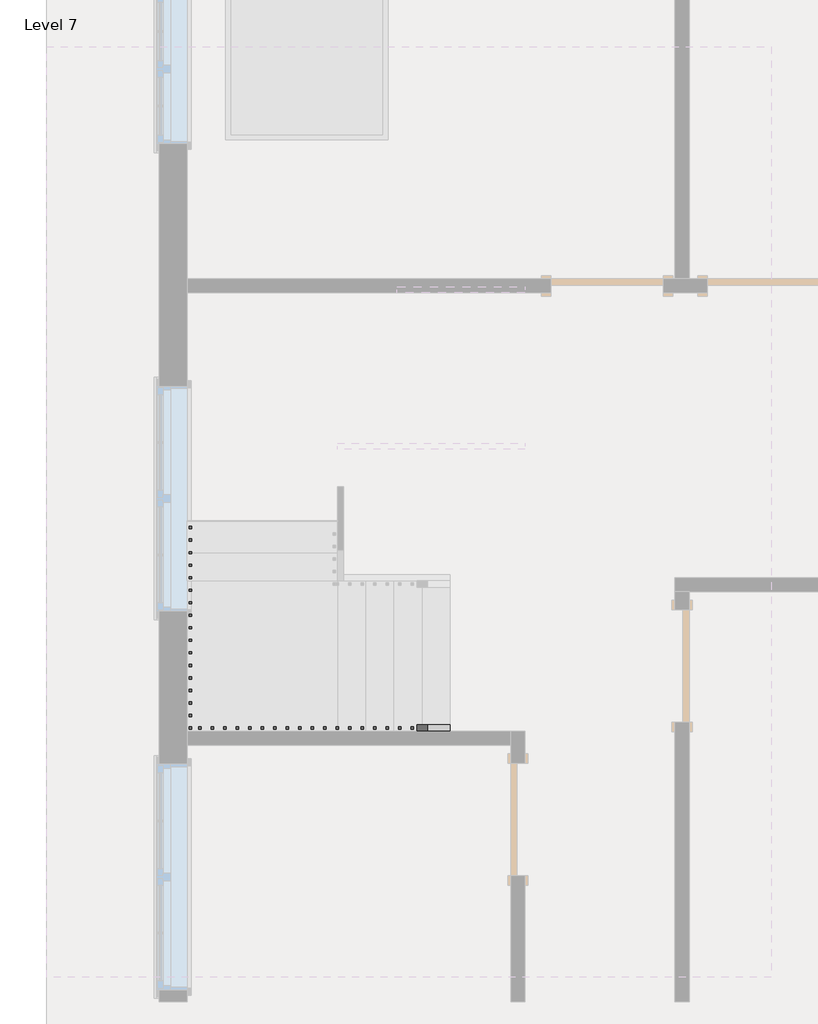
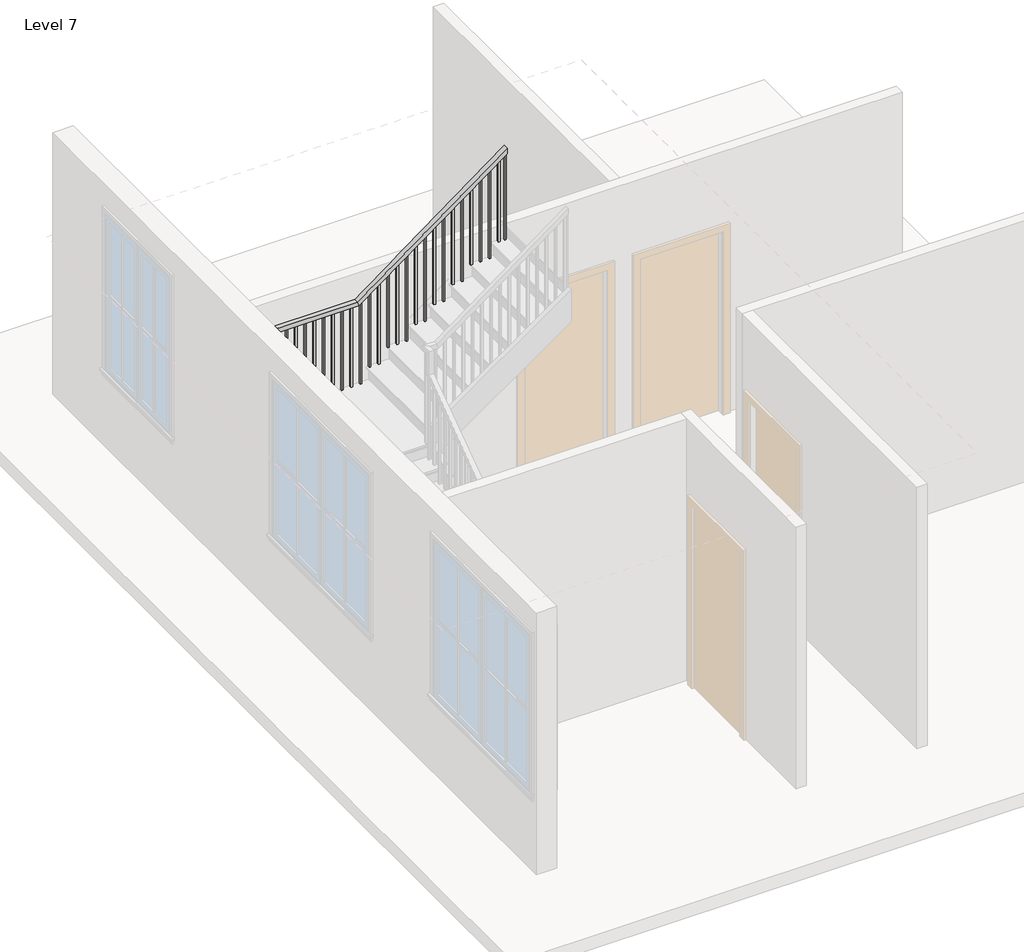
# One storey, part 2 of 3: 1 railing.
"""IFC4 building model written with IfcOpenShell, lengths in millimetres."""

from ifc_helpers import new_model, si_unit, frame, origin, place, context, project, spatial, polyline, outline, extrude, faceted_brep, element, save

model = new_model("IFC4")

# Units and contexts
model_context = context("Model", 3, world=origin())
ifc_project = project(units=[si_unit("LENGTHUNIT", "METRE", prefix="MILLI")], contexts=[model_context])

# Site, building, storey
site = spatial("IfcSite", under=ifc_project)
building = spatial("IfcBuilding", under=site)
storey = spatial("IfcBuildingStorey", under=building, Name="Level 7", Elevation=19050.0)

# Railing
placement = place(None, origin())
element("IfcRailing", 1, ObjectType="Handrail - Rectangular", at=placement, inside=storey, context=model_context, shape_type="SolidModel", body=[
    faceted_brep([(-2683.1105391, -2741.0373761, 20124.8210526), (-2683.1105391, -2741.0373761, 20062.7605986), (-2683.1105391, -2690.2373761, 20062.7605986), (-2683.1105391, -2690.2373761, 20124.8210526), (-3698.24463, -2741.0373761, 20837.1958533), (-3714.290777, -2741.0373761, 20786.3958533), (-3714.290777, -2690.2373761, 20786.3958533), (-3698.24463, -2690.2373761, 20837.1958533), (-4816.7105391, -2741.0373761, 20837.1958533), (-4816.7105391, -2741.0373761, 20786.3958533), (-4765.9105391, -2690.2373761, 20786.3958533), (-4765.9105391, -2690.2373761, 20837.1958533), (-4816.7105391, -1646.8618205, 20837.1958533), (-4816.7105391, -1630.5188912, 20786.3958533), (-4765.9105391, -1630.5188912, 20786.3958533), (-4765.9105391, -1646.8618205, 20837.1958533), (-4816.7105391, -308.3947094, 21797.8181818), (-4816.7105391, -292.0517801, 21747.0181818), (-4765.9105391, -292.0517801, 21747.0181818), (-4765.9105391, -308.3947094, 21797.8181818), (-4816.7105391, 814.9626239, 21797.8181818), (-4816.7105391, 814.9626239, 21747.0181818), (-4765.9105391, 764.1626239, 21747.0181818), (-4765.9105391, 764.1626239, 21797.8181818), (-3721.871578, 814.9626239, 21797.8181818), (-3705.1770744, 814.9626239, 21747.0181818), (-3705.1770744, 764.1626239, 21747.0181818), (-3721.871578, 764.1626239, 21797.8181818), (-2073.5105391, 814.9626239, 23012.4), (-2073.5105391, 764.1626239, 23012.4), (-2073.5105391, 764.1626239, 22949.2987868), (-2073.5105391, 814.9626239, 22949.2987868)], [[[0, 1, 2, 3]], [[1, 0, 4, 5]], [[2, 1, 5, 6]], [[3, 2, 6, 7]], [[0, 3, 7, 4]], [[5, 4, 8, 9]], [[6, 5, 9, 10]], [[7, 6, 10, 11]], [[4, 7, 11, 8]], [[9, 8, 12, 13]], [[10, 9, 13, 14]], [[11, 10, 14, 15]], [[8, 11, 15, 12]], [[13, 12, 16, 17]], [[14, 13, 17, 18]], [[15, 14, 18, 19]], [[12, 15, 19, 16]], [[17, 16, 20, 21]], [[18, 17, 21, 22]], [[19, 18, 22, 23]], [[16, 19, 23, 20]], [[21, 20, 24, 25]], [[22, 21, 25, 26]], [[23, 22, 26, 27]], [[20, 23, 27, 24]], [[28, 29, 30, 31]], [[25, 24, 28, 31]], [[26, 25, 31, 30]], [[27, 26, 30, 29]], [[24, 27, 29, 28]]]),
    extrude(outline(polyline([(22886.1329974, -2159.2355391), (21937.5789474, -2159.2355391), (21937.5789474, -2140.1855391), (22900.1698395, -2140.1855391), (22886.1329974, -2159.2355391)])), frame((0.0, 780.0376239, 0.0), z_axis=(0.0, 1.0, 0.0), x_axis=(0.0, 0.0, 1.0)), (0.0, 0.0, 1.0), 19.05),
    extrude(outline(polyline([(22811.2698395, -2260.8355391), (21777.1578947, -2260.8355391), (21777.1578947, -2241.7855391), (22825.3066816, -2241.7855391), (22811.2698395, -2260.8355391)])), frame((0.0, 780.0376239, 0.0), z_axis=(0.0, 1.0, 0.0), x_axis=(0.0, 0.0, 1.0)), (0.0, 0.0, 1.0), 19.05),
    extrude(outline(polyline([(22736.4066816, -2362.4355391), (21777.1578947, -2362.4355391), (21777.1578947, -2343.3855391), (22750.4435237, -2343.3855391), (22736.4066816, -2362.4355391)])), frame((0.0, 780.0376239, 0.0), z_axis=(0.0, 1.0, 0.0), x_axis=(0.0, 0.0, 1.0)), (0.0, 0.0, 1.0), 19.05),
    extrude(outline(polyline([(22661.5435237, -2464.0355391), (21777.1578947, -2464.0355391), (21777.1578947, -2444.9855391), (22675.5803658, -2444.9855391), (22661.5435237, -2464.0355391)])), frame((0.0, 780.0376239, 0.0), z_axis=(0.0, 1.0, 0.0), x_axis=(0.0, 0.0, 1.0)), (0.0, 0.0, 1.0), 19.05),
    extrude(outline(polyline([(22586.6803658, -2565.6355391), (21616.7368421, -2565.6355391), (21616.7368421, -2546.5855391), (22600.7172079, -2546.5855391), (22586.6803658, -2565.6355391)])), frame((0.0, 780.0376239, 0.0), z_axis=(0.0, 1.0, 0.0), x_axis=(0.0, 0.0, 1.0)), (0.0, 0.0, 1.0), 19.05),
    extrude(outline(polyline([(22511.8172079, -2667.2355391), (21616.7368421, -2667.2355391), (21616.7368421, -2648.1855391), (22525.85405, -2648.1855391), (22511.8172079, -2667.2355391)])), frame((0.0, 780.0376239, 0.0), z_axis=(0.0, 1.0, 0.0), x_axis=(0.0, 0.0, 1.0)), (0.0, 0.0, 1.0), 19.05),
    extrude(outline(polyline([(22436.95405, -2768.8355391), (21456.3157895, -2768.8355391), (21456.3157895, -2749.7855391), (22450.9908921, -2749.7855391), (22436.95405, -2768.8355391)])), frame((0.0, 780.0376239, 0.0), z_axis=(0.0, 1.0, 0.0), x_axis=(0.0, 0.0, 1.0)), (0.0, 0.0, 1.0), 19.05),
    extrude(outline(polyline([(22362.0908921, -2870.4355391), (21456.3157895, -2870.4355391), (21456.3157895, -2851.3855391), (22376.1277342, -2851.3855391), (22362.0908921, -2870.4355391)])), frame((0.0, 780.0376239, 0.0), z_axis=(0.0, 1.0, 0.0), x_axis=(0.0, 0.0, 1.0)), (0.0, 0.0, 1.0), 19.05),
    extrude(outline(polyline([(22287.2277342, -2972.0355391), (21295.8947368, -2972.0355391), (21295.8947368, -2952.9855391), (22301.2645763, -2952.9855391), (22287.2277342, -2972.0355391)])), frame((0.0, 780.0376239, 0.0), z_axis=(0.0, 1.0, 0.0), x_axis=(0.0, 0.0, 1.0)), (0.0, 0.0, 1.0), 19.05),
    extrude(outline(polyline([(22212.3645763, -3073.6355391), (21295.8947368, -3073.6355391), (21295.8947368, -3054.5855391), (22226.4014184, -3054.5855391), (22212.3645763, -3073.6355391)])), frame((0.0, 780.0376239, 0.0), z_axis=(0.0, 1.0, 0.0), x_axis=(0.0, 0.0, 1.0)), (0.0, 0.0, 1.0), 19.05),
    extrude(outline(polyline([(22137.5014184, -3175.2355391), (21135.4736842, -3175.2355391), (21135.4736842, -3156.1855391), (22151.5382605, -3156.1855391), (22137.5014184, -3175.2355391)])), frame((0.0, 780.0376239, 0.0), z_axis=(0.0, 1.0, 0.0), x_axis=(0.0, 0.0, 1.0)), (0.0, 0.0, 1.0), 19.05),
    extrude(outline(polyline([(22062.6382605, -3276.8355391), (21135.4736842, -3276.8355391), (21135.4736842, -3257.7855391), (22076.6751026, -3257.7855391), (22062.6382605, -3276.8355391)])), frame((0.0, 780.0376239, 0.0), z_axis=(0.0, 1.0, 0.0), x_axis=(0.0, 0.0, 1.0)), (0.0, 0.0, 1.0), 19.05),
    extrude(outline(polyline([(21987.7751026, -3378.4355391), (21135.4736842, -3378.4355391), (21135.4736842, -3359.3855391), (22001.8119447, -3359.3855391), (21987.7751026, -3378.4355391)])), frame((0.0, 780.0376239, 0.0), z_axis=(0.0, 1.0, 0.0), x_axis=(0.0, 0.0, 1.0)), (0.0, 0.0, 1.0), 19.05),
    extrude(outline(polyline([(21912.9119447, -3480.0355391), (20975.0526316, -3480.0355391), (20975.0526316, -3460.9855391), (21926.9487868, -3460.9855391), (21912.9119447, -3480.0355391)])), frame((0.0, 780.0376239, 0.0), z_axis=(0.0, 1.0, 0.0), x_axis=(0.0, 0.0, 1.0)), (0.0, 0.0, 1.0), 19.05),
    extrude(outline(polyline([(21838.0487868, -3581.6355391), (20975.0526316, -3581.6355391), (20975.0526316, -3562.5855391), (21852.0856289, -3562.5855391), (21838.0487868, -3581.6355391)])), frame((0.0, 780.0376239, 0.0), z_axis=(0.0, 1.0, 0.0), x_axis=(0.0, 0.0, 1.0)), (0.0, 0.0, 1.0), 19.05),
    extrude(outline(polyline([(21763.1856289, -3683.2355391), (20814.6315789, -3683.2355391), (20814.6315789, -3664.1855391), (21777.222471, -3664.1855391), (21763.1856289, -3683.2355391)])), frame((0.0, 780.0376239, 0.0), z_axis=(0.0, 1.0, 0.0), x_axis=(0.0, 0.0, 1.0)), (0.0, 0.0, 1.0), 19.05),
    extrude(outline(polyline([(-3784.8355391, 799.0876239), (-3765.7855391, 799.0876239), (-3765.7855391, 780.0376239), (-3784.8355391, 780.0376239), (-3784.8355391, 799.0876239)])), frame((0.0, 0.0, 20814.6315789), z_axis=(0.0, 0.0, 1.0), x_axis=(1.0, 0.0, 0.0)), (0.0, 0.0, 1.0), 932.3866029),
    extrude(outline(polyline([(-3886.4355391, 799.0876239), (-3867.3855391, 799.0876239), (-3867.3855391, 780.0376239), (-3886.4355391, 780.0376239), (-3886.4355391, 799.0876239)])), frame((0.0, 0.0, 20814.6315789), z_axis=(0.0, 0.0, 1.0), x_axis=(1.0, 0.0, 0.0)), (0.0, 0.0, 1.0), 932.3866029),
    extrude(outline(polyline([(-3988.0355391, 799.0876239), (-3968.9855391, 799.0876239), (-3968.9855391, 780.0376239), (-3988.0355391, 780.0376239), (-3988.0355391, 799.0876239)])), frame((0.0, 0.0, 20814.6315789), z_axis=(0.0, 0.0, 1.0), x_axis=(1.0, 0.0, 0.0)), (0.0, 0.0, 1.0), 932.3866029),
    extrude(outline(polyline([(-4089.6355391, 799.0876239), (-4070.5855391, 799.0876239), (-4070.5855391, 780.0376239), (-4089.6355391, 780.0376239), (-4089.6355391, 799.0876239)])), frame((0.0, 0.0, 20814.6315789), z_axis=(0.0, 0.0, 1.0), x_axis=(1.0, 0.0, 0.0)), (0.0, 0.0, 1.0), 932.3866029),
    extrude(outline(polyline([(-4191.2355391, 799.0876239), (-4172.1855391, 799.0876239), (-4172.1855391, 780.0376239), (-4191.2355391, 780.0376239), (-4191.2355391, 799.0876239)])), frame((0.0, 0.0, 20814.6315789), z_axis=(0.0, 0.0, 1.0), x_axis=(1.0, 0.0, 0.0)), (0.0, 0.0, 1.0), 932.3866029),
    extrude(outline(polyline([(-4292.8355391, 799.0876239), (-4273.7855391, 799.0876239), (-4273.7855391, 780.0376239), (-4292.8355391, 780.0376239), (-4292.8355391, 799.0876239)])), frame((0.0, 0.0, 20814.6315789), z_axis=(0.0, 0.0, 1.0), x_axis=(1.0, 0.0, 0.0)), (0.0, 0.0, 1.0), 932.3866029),
    extrude(outline(polyline([(-4394.4355391, 799.0876239), (-4375.3855391, 799.0876239), (-4375.3855391, 780.0376239), (-4394.4355391, 780.0376239), (-4394.4355391, 799.0876239)])), frame((0.0, 0.0, 20814.6315789), z_axis=(0.0, 0.0, 1.0), x_axis=(1.0, 0.0, 0.0)), (0.0, 0.0, 1.0), 932.3866029),
    extrude(outline(polyline([(-4496.0355391, 799.0876239), (-4476.9855391, 799.0876239), (-4476.9855391, 780.0376239), (-4496.0355391, 780.0376239), (-4496.0355391, 799.0876239)])), frame((0.0, 0.0, 20814.6315789), z_axis=(0.0, 0.0, 1.0), x_axis=(1.0, 0.0, 0.0)), (0.0, 0.0, 1.0), 932.3866029),
    extrude(outline(polyline([(-4597.6355391, 799.0876239), (-4578.5855391, 799.0876239), (-4578.5855391, 780.0376239), (-4597.6355391, 780.0376239), (-4597.6355391, 799.0876239)])), frame((0.0, 0.0, 20814.6315789), z_axis=(0.0, 0.0, 1.0), x_axis=(1.0, 0.0, 0.0)), (0.0, 0.0, 1.0), 932.3866029),
    extrude(outline(polyline([(-4699.2355391, 799.0876239), (-4680.1855391, 799.0876239), (-4680.1855391, 780.0376239), (-4699.2355391, 780.0376239), (-4699.2355391, 799.0876239)])), frame((0.0, 0.0, 20814.6315789), z_axis=(0.0, 0.0, 1.0), x_axis=(1.0, 0.0, 0.0)), (0.0, 0.0, 1.0), 932.3866029),
    extrude(outline(polyline([(-4800.8355391, 729.2376239), (-4800.8355391, 748.2876239), (-4781.7855391, 748.2876239), (-4781.7855391, 729.2376239), (-4800.8355391, 729.2376239)])), frame((0.0, 0.0, 20814.6315789), z_axis=(0.0, 0.0, 1.0), x_axis=(1.0, 0.0, 0.0)), (0.0, 0.0, 1.0), 932.3866029),
    extrude(outline(polyline([(-4800.8355391, 627.6376239), (-4800.8355391, 646.6876239), (-4781.7855391, 646.6876239), (-4781.7855391, 627.6376239), (-4800.8355391, 627.6376239)])), frame((0.0, 0.0, 20814.6315789), z_axis=(0.0, 0.0, 1.0), x_axis=(1.0, 0.0, 0.0)), (0.0, 0.0, 1.0), 932.3866029),
    extrude(outline(polyline([(-4800.8355391, 526.0376239), (-4800.8355391, 545.0876239), (-4781.7855391, 545.0876239), (-4781.7855391, 526.0376239), (-4800.8355391, 526.0376239)])), frame((0.0, 0.0, 20814.6315789), z_axis=(0.0, 0.0, 1.0), x_axis=(1.0, 0.0, 0.0)), (0.0, 0.0, 1.0), 932.3866029),
    extrude(outline(polyline([(-4800.8355391, 424.4376239), (-4800.8355391, 443.4876239), (-4781.7855391, 443.4876239), (-4781.7855391, 424.4376239), (-4800.8355391, 424.4376239)])), frame((0.0, 0.0, 20814.6315789), z_axis=(0.0, 0.0, 1.0), x_axis=(1.0, 0.0, 0.0)), (0.0, 0.0, 1.0), 932.3866029),
    extrude(outline(polyline([(-4800.8355391, 322.8376239), (-4800.8355391, 341.8876239), (-4781.7855391, 341.8876239), (-4781.7855391, 322.8376239), (-4800.8355391, 322.8376239)])), frame((0.0, 0.0, 20814.6315789), z_axis=(0.0, 0.0, 1.0), x_axis=(1.0, 0.0, 0.0)), (0.0, 0.0, 1.0), 932.3866029),
    extrude(outline(polyline([(-4800.8355391, 221.2376239), (-4800.8355391, 240.2876239), (-4781.7855391, 240.2876239), (-4781.7855391, 221.2376239), (-4800.8355391, 221.2376239)])), frame((0.0, 0.0, 20814.6315789), z_axis=(0.0, 0.0, 1.0), x_axis=(1.0, 0.0, 0.0)), (0.0, 0.0, 1.0), 932.3866029),
    extrude(outline(polyline([(-4800.8355391, 119.6376239), (-4800.8355391, 138.6876239), (-4781.7855391, 138.6876239), (-4781.7855391, 119.6376239), (-4800.8355391, 119.6376239)])), frame((0.0, 0.0, 20814.6315789), z_axis=(0.0, 0.0, 1.0), x_axis=(1.0, 0.0, 0.0)), (0.0, 0.0, 1.0), 932.3866029),
    extrude(outline(polyline([(-4800.8355391, 18.0376239), (-4800.8355391, 37.0876239), (-4781.7855391, 37.0876239), (-4781.7855391, 18.0376239), (-4800.8355391, 18.0376239)])), frame((0.0, 0.0, 20814.6315789), z_axis=(0.0, 0.0, 1.0), x_axis=(1.0, 0.0, 0.0)), (0.0, 0.0, 1.0), 932.3866029),
    extrude(outline(polyline([(-4800.8355391, -83.5623761), (-4800.8355391, -64.5123761), (-4781.7855391, -64.5123761), (-4781.7855391, -83.5623761), (-4800.8355391, -83.5623761)])), frame((0.0, 0.0, 20814.6315789), z_axis=(0.0, 0.0, 1.0), x_axis=(1.0, 0.0, 0.0)), (0.0, 0.0, 1.0), 932.3866029),
    extrude(outline(polyline([(-4800.8355391, -185.1623761), (-4800.8355391, -166.1123761), (-4781.7855391, -166.1123761), (-4781.7855391, -185.1623761), (-4800.8355391, -185.1623761)])), frame((0.0, 0.0, 20814.6315789), z_axis=(0.0, 0.0, 1.0), x_axis=(1.0, 0.0, 0.0)), (0.0, 0.0, 1.0), 932.3866029),
    extrude(outline(polyline([(-4800.8355391, -286.7623761), (-4800.8355391, -267.7123761), (-4781.7855391, -267.7123761), (-4781.7855391, -286.7623761), (-4800.8355391, -286.7623761)])), frame((0.0, 0.0, 20814.6315789), z_axis=(0.0, 0.0, 1.0), x_axis=(1.0, 0.0, 0.0)), (0.0, 0.0, 1.0), 932.3866029),
    extrude(outline(polyline([(-369.3123761, 21691.5679933), (-369.3123761, 20814.6315789), (-388.3623761, 20814.6315789), (-388.3623761, 21677.8957445), (-369.3123761, 21691.5679933)])), frame((-4800.8355391, 0.0, 0.0), z_axis=(1.0, 0.0, 0.0), x_axis=(0.0, 1.0, 0.0)), (0.0, 0.0, 1.0), 19.05),
    extrude(outline(polyline([(-470.9123761, 21618.649333), (-470.9123761, 20654.2105263), (-489.9623761, 20654.2105263), (-489.9623761, 21604.9770842), (-470.9123761, 21618.649333)])), frame((-4800.8355391, 0.0, 0.0), z_axis=(1.0, 0.0, 0.0), x_axis=(0.0, 1.0, 0.0)), (0.0, 0.0, 1.0), 19.05),
    extrude(outline(polyline([(-572.5123761, 21545.7306727), (-572.5123761, 20654.2105263), (-591.5623761, 20654.2105263), (-591.5623761, 21532.0584239), (-572.5123761, 21545.7306727)])), frame((-4800.8355391, 0.0, 0.0), z_axis=(1.0, 0.0, 0.0), x_axis=(0.0, 1.0, 0.0)), (0.0, 0.0, 1.0), 19.05),
    extrude(outline(polyline([(-674.1123761, 21472.8120124), (-674.1123761, 20493.7894737), (-693.1623761, 20493.7894737), (-693.1623761, 21459.1397636), (-674.1123761, 21472.8120124)])), frame((-4800.8355391, 0.0, 0.0), z_axis=(1.0, 0.0, 0.0), x_axis=(0.0, 1.0, 0.0)), (0.0, 0.0, 1.0), 19.05),
    extrude(outline(polyline([(-775.7123761, 21399.8933521), (-775.7123761, 20493.7894737), (-794.7623761, 20493.7894737), (-794.7623761, 21386.2211033), (-775.7123761, 21399.8933521)])), frame((-4800.8355391, 0.0, 0.0), z_axis=(1.0, 0.0, 0.0), x_axis=(0.0, 1.0, 0.0)), (0.0, 0.0, 1.0), 19.05),
    extrude(outline(polyline([(-877.3123761, 21326.9746919), (-877.3123761, 20333.3684211), (-896.3623761, 20333.3684211), (-896.3623761, 21313.302443), (-877.3123761, 21326.9746919)])), frame((-4800.8355391, 0.0, 0.0), z_axis=(1.0, 0.0, 0.0), x_axis=(0.0, 1.0, 0.0)), (0.0, 0.0, 1.0), 19.05),
    extrude(outline(polyline([(-978.9123761, 21254.0560316), (-978.9123761, 20333.3684211), (-997.9623761, 20333.3684211), (-997.9623761, 21240.3837828), (-978.9123761, 21254.0560316)])), frame((-4800.8355391, 0.0, 0.0), z_axis=(1.0, 0.0, 0.0), x_axis=(0.0, 1.0, 0.0)), (0.0, 0.0, 1.0), 19.05),
    extrude(outline(polyline([(-1080.5123761, 21181.1373713), (-1080.5123761, 20172.9473684), (-1099.5623761, 20172.9473684), (-1099.5623761, 21167.4651225), (-1080.5123761, 21181.1373713)])), frame((-4800.8355391, 0.0, 0.0), z_axis=(1.0, 0.0, 0.0), x_axis=(0.0, 1.0, 0.0)), (0.0, 0.0, 1.0), 19.05),
    extrude(outline(polyline([(-1182.1123761, 21108.218711), (-1182.1123761, 20172.9473684), (-1201.1623761, 20172.9473684), (-1201.1623761, 21094.5464622), (-1182.1123761, 21108.218711)])), frame((-4800.8355391, 0.0, 0.0), z_axis=(1.0, 0.0, 0.0), x_axis=(0.0, 1.0, 0.0)), (0.0, 0.0, 1.0), 19.05),
    extrude(outline(polyline([(-1283.7123761, 21035.3000507), (-1283.7123761, 20172.9473684), (-1302.7623761, 20172.9473684), (-1302.7623761, 21021.6278019), (-1283.7123761, 21035.3000507)])), frame((-4800.8355391, 0.0, 0.0), z_axis=(1.0, 0.0, 0.0), x_axis=(0.0, 1.0, 0.0)), (0.0, 0.0, 1.0), 19.05),
    extrude(outline(polyline([(-1385.3123761, 20962.3813904), (-1385.3123761, 20012.5263158), (-1404.3623761, 20012.5263158), (-1404.3623761, 20948.7091416), (-1385.3123761, 20962.3813904)])), frame((-4800.8355391, 0.0, 0.0), z_axis=(1.0, 0.0, 0.0), x_axis=(0.0, 1.0, 0.0)), (0.0, 0.0, 1.0), 19.05),
    extrude(outline(polyline([(-1486.9123761, 20889.4627301), (-1486.9123761, 20012.5263158), (-1505.9623761, 20012.5263158), (-1505.9623761, 20875.7904813), (-1486.9123761, 20889.4627301)])), frame((-4800.8355391, 0.0, 0.0), z_axis=(1.0, 0.0, 0.0), x_axis=(0.0, 1.0, 0.0)), (0.0, 0.0, 1.0), 19.05),
    extrude(outline(polyline([(-1588.5123761, 20816.5440698), (-1588.5123761, 19852.1052632), (-1607.5623761, 19852.1052632), (-1607.5623761, 20802.871821), (-1588.5123761, 20816.5440698)])), frame((-4800.8355391, 0.0, 0.0), z_axis=(1.0, 0.0, 0.0), x_axis=(0.0, 1.0, 0.0)), (0.0, 0.0, 1.0), 19.05),
    extrude(outline(polyline([(-4800.8355391, -1709.1623761), (-4800.8355391, -1690.1123761), (-4781.7855391, -1690.1123761), (-4781.7855391, -1709.1623761), (-4800.8355391, -1709.1623761)])), frame((0.0, 0.0, 19852.1052632), z_axis=(0.0, 0.0, 1.0), x_axis=(1.0, 0.0, 0.0)), (0.0, 0.0, 1.0), 934.2905901),
    extrude(outline(polyline([(-4800.8355391, -1810.7623761), (-4800.8355391, -1791.7123761), (-4781.7855391, -1791.7123761), (-4781.7855391, -1810.7623761), (-4800.8355391, -1810.7623761)])), frame((0.0, 0.0, 19852.1052632), z_axis=(0.0, 0.0, 1.0), x_axis=(1.0, 0.0, 0.0)), (0.0, 0.0, 1.0), 934.2905901),
    extrude(outline(polyline([(-4800.8355391, -1912.3623761), (-4800.8355391, -1893.3123761), (-4781.7855391, -1893.3123761), (-4781.7855391, -1912.3623761), (-4800.8355391, -1912.3623761)])), frame((0.0, 0.0, 19852.1052632), z_axis=(0.0, 0.0, 1.0), x_axis=(1.0, 0.0, 0.0)), (0.0, 0.0, 1.0), 934.2905901),
    extrude(outline(polyline([(-4800.8355391, -2013.9623761), (-4800.8355391, -1994.9123761), (-4781.7855391, -1994.9123761), (-4781.7855391, -2013.9623761), (-4800.8355391, -2013.9623761)])), frame((0.0, 0.0, 19852.1052632), z_axis=(0.0, 0.0, 1.0), x_axis=(1.0, 0.0, 0.0)), (0.0, 0.0, 1.0), 934.2905901),
    extrude(outline(polyline([(-4800.8355391, -2115.5623761), (-4800.8355391, -2096.5123761), (-4781.7855391, -2096.5123761), (-4781.7855391, -2115.5623761), (-4800.8355391, -2115.5623761)])), frame((0.0, 0.0, 19852.1052632), z_axis=(0.0, 0.0, 1.0), x_axis=(1.0, 0.0, 0.0)), (0.0, 0.0, 1.0), 934.2905901),
    extrude(outline(polyline([(-4800.8355391, -2217.1623761), (-4800.8355391, -2198.1123761), (-4781.7855391, -2198.1123761), (-4781.7855391, -2217.1623761), (-4800.8355391, -2217.1623761)])), frame((0.0, 0.0, 19852.1052632), z_axis=(0.0, 0.0, 1.0), x_axis=(1.0, 0.0, 0.0)), (0.0, 0.0, 1.0), 934.2905901),
    extrude(outline(polyline([(-4800.8355391, -2318.7623761), (-4800.8355391, -2299.7123761), (-4781.7855391, -2299.7123761), (-4781.7855391, -2318.7623761), (-4800.8355391, -2318.7623761)])), frame((0.0, 0.0, 19852.1052632), z_axis=(0.0, 0.0, 1.0), x_axis=(1.0, 0.0, 0.0)), (0.0, 0.0, 1.0), 934.2905901),
    extrude(outline(polyline([(-4800.8355391, -2420.3623761), (-4800.8355391, -2401.3123761), (-4781.7855391, -2401.3123761), (-4781.7855391, -2420.3623761), (-4800.8355391, -2420.3623761)])), frame((0.0, 0.0, 19852.1052632), z_axis=(0.0, 0.0, 1.0), x_axis=(1.0, 0.0, 0.0)), (0.0, 0.0, 1.0), 934.2905901),
    extrude(outline(polyline([(-4800.8355391, -2521.9623761), (-4800.8355391, -2502.9123761), (-4781.7855391, -2502.9123761), (-4781.7855391, -2521.9623761), (-4800.8355391, -2521.9623761)])), frame((0.0, 0.0, 19852.1052632), z_axis=(0.0, 0.0, 1.0), x_axis=(1.0, 0.0, 0.0)), (0.0, 0.0, 1.0), 934.2905901),
    extrude(outline(polyline([(-4800.8355391, -2623.5623761), (-4800.8355391, -2604.5123761), (-4781.7855391, -2604.5123761), (-4781.7855391, -2623.5623761), (-4800.8355391, -2623.5623761)])), frame((0.0, 0.0, 19852.1052632), z_axis=(0.0, 0.0, 1.0), x_axis=(1.0, 0.0, 0.0)), (0.0, 0.0, 1.0), 934.2905901),
    extrude(outline(polyline([(-4705.5855391, -2725.1623761), (-4724.6355391, -2725.1623761), (-4724.6355391, -2706.1123761), (-4705.5855391, -2706.1123761), (-4705.5855391, -2725.1623761)])), frame((0.0, 0.0, 19852.1052632), z_axis=(0.0, 0.0, 1.0), x_axis=(1.0, 0.0, 0.0)), (0.0, 0.0, 1.0), 934.2905901),
    extrude(outline(polyline([(-4603.9855391, -2725.1623761), (-4623.0355391, -2725.1623761), (-4623.0355391, -2706.1123761), (-4603.9855391, -2706.1123761), (-4603.9855391, -2725.1623761)])), frame((0.0, 0.0, 19852.1052632), z_axis=(0.0, 0.0, 1.0), x_axis=(1.0, 0.0, 0.0)), (0.0, 0.0, 1.0), 934.2905901),
    extrude(outline(polyline([(-4502.3855391, -2725.1623761), (-4521.4355391, -2725.1623761), (-4521.4355391, -2706.1123761), (-4502.3855391, -2706.1123761), (-4502.3855391, -2725.1623761)])), frame((0.0, 0.0, 19852.1052632), z_axis=(0.0, 0.0, 1.0), x_axis=(1.0, 0.0, 0.0)), (0.0, 0.0, 1.0), 934.2905901),
    extrude(outline(polyline([(-4400.7855391, -2725.1623761), (-4419.8355391, -2725.1623761), (-4419.8355391, -2706.1123761), (-4400.7855391, -2706.1123761), (-4400.7855391, -2725.1623761)])), frame((0.0, 0.0, 19852.1052632), z_axis=(0.0, 0.0, 1.0), x_axis=(1.0, 0.0, 0.0)), (0.0, 0.0, 1.0), 934.2905901),
    extrude(outline(polyline([(-4299.1855391, -2725.1623761), (-4318.2355391, -2725.1623761), (-4318.2355391, -2706.1123761), (-4299.1855391, -2706.1123761), (-4299.1855391, -2725.1623761)])), frame((0.0, 0.0, 19852.1052632), z_axis=(0.0, 0.0, 1.0), x_axis=(1.0, 0.0, 0.0)), (0.0, 0.0, 1.0), 934.2905901),
    extrude(outline(polyline([(-4197.5855391, -2725.1623761), (-4216.6355391, -2725.1623761), (-4216.6355391, -2706.1123761), (-4197.5855391, -2706.1123761), (-4197.5855391, -2725.1623761)])), frame((0.0, 0.0, 19852.1052632), z_axis=(0.0, 0.0, 1.0), x_axis=(1.0, 0.0, 0.0)), (0.0, 0.0, 1.0), 934.2905901),
    extrude(outline(polyline([(-4095.9855391, -2725.1623761), (-4115.0355391, -2725.1623761), (-4115.0355391, -2706.1123761), (-4095.9855391, -2706.1123761), (-4095.9855391, -2725.1623761)])), frame((0.0, 0.0, 19852.1052632), z_axis=(0.0, 0.0, 1.0), x_axis=(1.0, 0.0, 0.0)), (0.0, 0.0, 1.0), 934.2905901),
    extrude(outline(polyline([(-3994.3855391, -2725.1623761), (-4013.4355391, -2725.1623761), (-4013.4355391, -2706.1123761), (-3994.3855391, -2706.1123761), (-3994.3855391, -2725.1623761)])), frame((0.0, 0.0, 19852.1052632), z_axis=(0.0, 0.0, 1.0), x_axis=(1.0, 0.0, 0.0)), (0.0, 0.0, 1.0), 934.2905901),
    extrude(outline(polyline([(-3892.7855391, -2725.1623761), (-3911.8355391, -2725.1623761), (-3911.8355391, -2706.1123761), (-3892.7855391, -2706.1123761), (-3892.7855391, -2725.1623761)])), frame((0.0, 0.0, 19852.1052632), z_axis=(0.0, 0.0, 1.0), x_axis=(1.0, 0.0, 0.0)), (0.0, 0.0, 1.0), 934.2905901),
    extrude(outline(polyline([(-3791.1855391, -2725.1623761), (-3810.2355391, -2725.1623761), (-3810.2355391, -2706.1123761), (-3791.1855391, -2706.1123761), (-3791.1855391, -2725.1623761)])), frame((0.0, 0.0, 19852.1052632), z_axis=(0.0, 0.0, 1.0), x_axis=(1.0, 0.0, 0.0)), (0.0, 0.0, 1.0), 934.2905901),
    extrude(outline(polyline([(-3689.5855391, -2725.1623761), (-3708.6355391, -2725.1623761), (-3708.6355391, -2706.1123761), (-3689.5855391, -2706.1123761), (-3689.5855391, -2725.1623761)])), frame((0.0, 0.0, 19852.1052632), z_axis=(0.0, 0.0, 1.0), x_axis=(1.0, 0.0, 0.0)), (0.0, 0.0, 1.0), 934.2905901),
    extrude(outline(polyline([(20711.1290196, -3607.0355391), (19852.1052632, -3607.0355391), (19852.1052632, -3587.9855391), (20697.7605986, -3587.9855391), (20711.1290196, -3607.0355391)])), frame((0.0, -2725.1623761, 0.0), z_axis=(0.0, 1.0, 0.0), x_axis=(0.0, 0.0, 1.0)), (0.0, 0.0, 1.0), 19.05),
    extrude(outline(polyline([(20639.830774, -3505.4355391), (19691.6842105, -3505.4355391), (19691.6842105, -3486.3855391), (20626.462353, -3486.3855391), (20639.830774, -3505.4355391)])), frame((0.0, -2725.1623761, 0.0), z_axis=(0.0, 1.0, 0.0), x_axis=(0.0, 0.0, 1.0)), (0.0, 0.0, 1.0), 19.05),
    extrude(outline(polyline([(20568.5325284, -3403.8355391), (19691.6842105, -3403.8355391), (19691.6842105, -3384.7855391), (20555.1641074, -3384.7855391), (20568.5325284, -3403.8355391)])), frame((0.0, -2725.1623761, 0.0), z_axis=(0.0, 1.0, 0.0), x_axis=(0.0, 0.0, 1.0)), (0.0, 0.0, 1.0), 19.05),
    extrude(outline(polyline([(20497.2342828, -3302.2355391), (19531.2631579, -3302.2355391), (19531.2631579, -3283.1855391), (20483.8658617, -3283.1855391), (20497.2342828, -3302.2355391)])), frame((0.0, -2725.1623761, 0.0), z_axis=(0.0, 1.0, 0.0), x_axis=(0.0, 0.0, 1.0)), (0.0, 0.0, 1.0), 19.05),
    extrude(outline(polyline([(20425.9360372, -3200.6355391), (19531.2631579, -3200.6355391), (19531.2631579, -3181.5855391), (20412.5676161, -3181.5855391), (20425.9360372, -3200.6355391)])), frame((0.0, -2725.1623761, 0.0), z_axis=(0.0, 1.0, 0.0), x_axis=(0.0, 0.0, 1.0)), (0.0, 0.0, 1.0), 19.05),
    extrude(outline(polyline([(20354.6377916, -3099.0355391), (19370.8421053, -3099.0355391), (19370.8421053, -3079.9855391), (20341.2693705, -3079.9855391), (20354.6377916, -3099.0355391)])), frame((0.0, -2725.1623761, 0.0), z_axis=(0.0, 1.0, 0.0), x_axis=(0.0, 0.0, 1.0)), (0.0, 0.0, 1.0), 19.05),
    extrude(outline(polyline([(20283.3395459, -2997.4355391), (19370.8421053, -2997.4355391), (19370.8421053, -2978.3855391), (20269.9711249, -2978.3855391), (20283.3395459, -2997.4355391)])), frame((0.0, -2725.1623761, 0.0), z_axis=(0.0, 1.0, 0.0), x_axis=(0.0, 0.0, 1.0)), (0.0, 0.0, 1.0), 19.05),
    extrude(outline(polyline([(20212.0413003, -2895.8355391), (19210.4210526, -2895.8355391), (19210.4210526, -2876.7855391), (20198.6728793, -2876.7855391), (20212.0413003, -2895.8355391)])), frame((0.0, -2725.1623761, 0.0), z_axis=(0.0, 1.0, 0.0), x_axis=(0.0, 0.0, 1.0)), (0.0, 0.0, 1.0), 19.05),
    extrude(outline(polyline([(20140.7430547, -2794.2355391), (19210.4210526, -2794.2355391), (19210.4210526, -2775.1855391), (20127.3746337, -2775.1855391), (20140.7430547, -2794.2355391)])), frame((0.0, -2725.1623761, 0.0), z_axis=(0.0, 1.0, 0.0), x_axis=(0.0, 0.0, 1.0)), (0.0, 0.0, 1.0), 19.05),
    extrude(outline(polyline([(-4800.8355391, 780.0376239), (-4800.8355391, 799.0876239), (-4781.7855391, 799.0876239), (-4781.7855391, 780.0376239), (-4800.8355391, 780.0376239)])), frame((0.0, 0.0, 20814.6315789), z_axis=(0.0, 0.0, 1.0), x_axis=(1.0, 0.0, 0.0)), (0.0, 0.0, 1.0), 932.3866029),
    extrude(outline(polyline([(-4781.7855391, -2725.1623761), (-4800.8355391, -2725.1623761), (-4800.8355391, -2706.1123761), (-4781.7855391, -2706.1123761), (-4781.7855391, -2725.1623761)])), frame((0.0, 0.0, 19852.1052632), z_axis=(0.0, 0.0, 1.0), x_axis=(1.0, 0.0, 0.0)), (0.0, 0.0, 1.0), 934.2905901),
    extrude(outline(polyline([(22935.2619447, -2092.5605391), (21937.5789474, -2092.5605391), (21937.5789474, -2073.5105391), (22949.2987868, -2073.5105391), (22935.2619447, -2092.5605391)])), frame((0.0, 780.0376239, 0.0), z_axis=(0.0, 1.0, 0.0), x_axis=(0.0, 0.0, 1.0)), (0.0, 0.0, 1.0), 19.05),
    extrude(outline(polyline([(20076.1290196, -2702.1605391), (19210.4210526, -2702.1605391), (19210.4210526, -2683.1105391), (20062.7605986, -2683.1105391), (20076.1290196, -2702.1605391)])), frame((0.0, -2725.1623761, 0.0), z_axis=(0.0, 1.0, 0.0), x_axis=(0.0, 0.0, 1.0)), (0.0, 0.0, 1.0), 19.05),
])

save(model, "model.ifc")

# Revit data of these elements
# Type "Handrail - Rectangular"
#   Assembly Code = "C2010400"
#   built-in parameter 1008612 = 0.0416667 (stored number, unit not read)
#   built-in parameter 1008611 = 0.0416667 (stored number, unit not read)
#   built-in parameter 1008609 = 0.333333 (stored number, unit not read)
#   built-in parameter 1008604 = 0.166667 (stored number, unit not read)
#   built-in parameter 1008603 = 0.166667 (stored number, unit not read)
#   Railing Height = 3' - 0"
#   built-in parameter 1008630 = 2
#   built-in parameter 1008610 = 2
#   built-in parameter 1008618 = Baluster - Square : 3/4"
# Element 1 (IfcRailing, "Handrail - Rectangular")
#   Phase Created = New Construction
